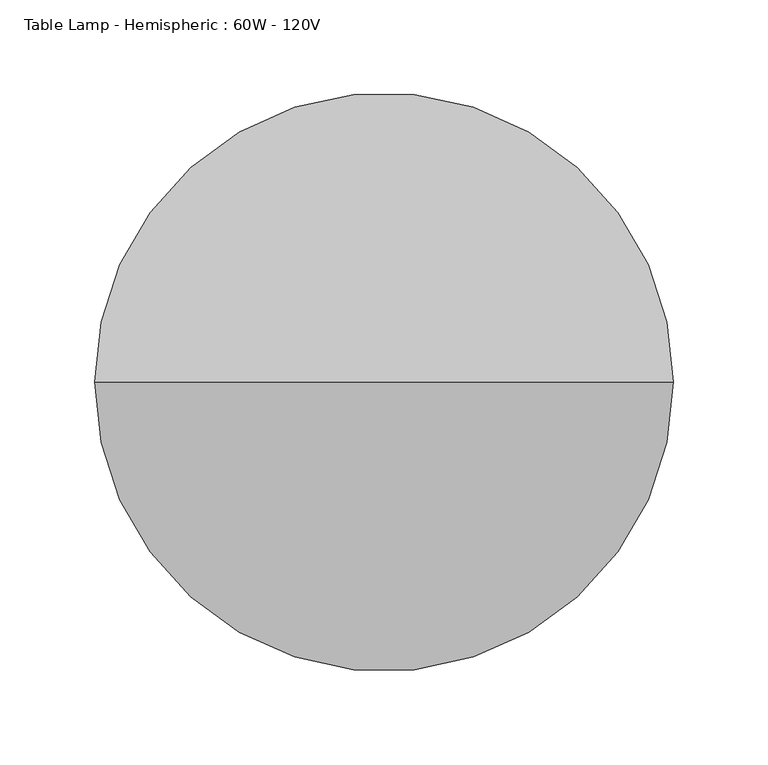
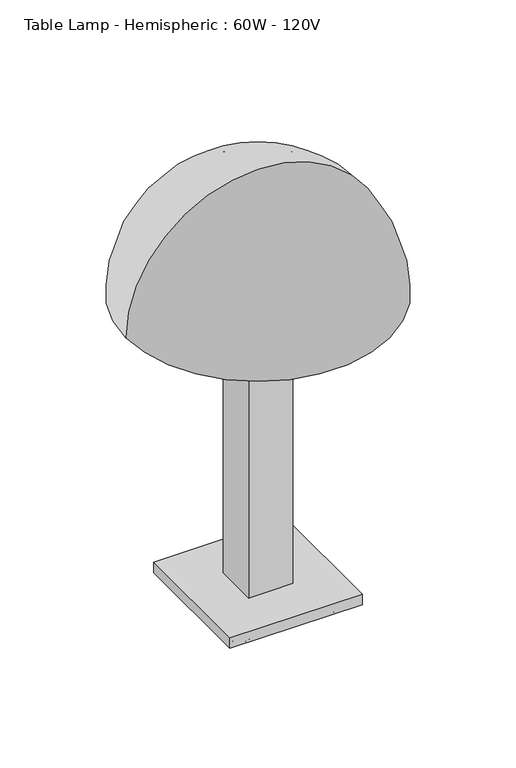
"""IFC4 building model written with IfcOpenShell, lengths in millimetres: light fixture geometry, Table Lamp - Hemispheric : 60W - 120V."""

from ifc_helpers import new_model, si_unit, point, frame, origin, origin_2d, place, context, project, spatial, polyline, circle_curve, ellipse_curve, trimmed, segment, composite_curve, outline, extrude, source, transform, mapped, element, save
from ifc_brep_helpers import plane_surface, revolved_surface, advanced_brep


def table_lamp_hemispheric_60w_120v_02721d88(model_context):
    return source(origin(), model_context, "Body", "SolidModel", [
        advanced_brep(
        [(0.0, 0.0, 524.5095504), (152.4, 0.0, 372.1095504), (-152.4, 0.0, 372.1095504), (-146.05, 0.0, 372.1095504), (146.05, 0.0, 372.1095504), (0.0, 0.0, 518.1595504)],
        [
            (0, 1, circle_curve(frame((0.0, 0.0, 372.1095504), z_axis=(0.0, 1.0, 0.0), x_axis=(1.0, 0.0, 0.0)), 152.4)),
            (1, 2, circle_curve(frame((0.0, 0.0, 372.1095504), z_axis=(0.0, 0.0, 1.0), x_axis=(1.0, 0.0, 0.0)), 152.4)),
            (2, 0, circle_curve(frame((0.0, 0.0, 372.1095504), z_axis=(0.0, 1.0, 0.0), x_axis=(-1.0, 0.0, 0.0)), 152.4)),
            (2, 1, circle_curve(frame((0.0, 0.0, 372.1095504), z_axis=(0.0, 0.0, 1.0), x_axis=(1.0, 0.0, 0.0)), 152.4)),
            (3, 4, circle_curve(frame((0.0, 0.0, 372.1095504), z_axis=(0.0, 0.0, -1.0), x_axis=(1.0, 0.0, 0.0)), 146.05)),
            (4, 5, circle_curve(frame((0.0, 0.0, 372.1095504), z_axis=(0.0, -1.0, 0.0), x_axis=(1.0, 0.0, 0.0)), 146.05)),
            (5, 3, circle_curve(frame((0.0, 0.0, 372.1095504), z_axis=(0.0, -1.0, 0.0), x_axis=(-1.0, 0.0, 0.0)), 146.05)),
            (4, 3, circle_curve(frame((0.0, 0.0, 372.1095504), z_axis=(0.0, 0.0, -1.0), x_axis=(1.0, 0.0, 0.0)), 146.05)),
            (1, 4),
            (3, 2),
        ],
        [
            revolved_surface(trimmed(ellipse_curve(frame((0.0, 0.0, 372.1095504), z_axis=(0.0, -1.0, 0.0), x_axis=(1.0, 0.0, 0.0)), 152.4, 152.4), [point((152.4, 0.0, 372.1095504))], [point((0.0, 0.0, 524.5095504))], True, "CARTESIAN"), (0.0, 0.0, 552.6321699), (0.0, 0.0, 1.0)),
            revolved_surface(trimmed(ellipse_curve(frame((0.0, 0.0, 372.1095504), z_axis=(0.0, 1.0, 0.0), x_axis=(1.0, 0.0, 0.0)), 146.05, 146.05), [point((0.0, 0.0, 518.1595504))], [point((146.05, 0.0, 372.1095504))], True, "CARTESIAN"), (0.0, 0.0, 552.6321699), (0.0, 0.0, 1.0)),
            plane_surface(frame((0.0, 0.0, 372.1095504), z_axis=(0.0, 0.0, -1.0), x_axis=(1.0, 0.0, 0.0))),
        ],
        [
            (0, [[1, 2, 3]]),
            (0, [[-3, 4, -1]]),
            (1, [[5, 6, 7]]),
            (1, [[8, -7, -6]]),
            (2, [[-2, 9, -5, 10]]),
            (2, [[-4, -10, -8, -9]]),
        ],
    ),
        extrude(outline(composite_curve([segment(trimmed(circle_curve(origin_2d(), 6.35), [point((-6.35, 0.0))], [point((6.35, 0.0))], False, "CARTESIAN"), True, "CONTINUOUS"), segment(trimmed(circle_curve(origin_2d(), 6.35), [point((6.35, 0.0))], [point((-6.35, 0.0))], False, "CARTESIAN"), True, "CONTINUOUS")], self_intersect=False)), frame((0.0, 0.0, 330.2), z_axis=(0.0, 0.0, 1.0), x_axis=(1.0, 0.0, 0.0)), (0.0, 0.0, 1.0), 63.5),
        extrude(outline(polyline([(25.4, -25.4), (-25.4, -25.4), (-25.4, 25.4), (25.4, 25.4), (25.4, -25.4)])), frame((0.0, 0.0, 25.4), z_axis=(0.0, 0.0, 1.0), x_axis=(1.0, 0.0, 0.0)), (0.0, 0.0, 1.0), 304.8),
        advanced_brep(
        [(-66.7336963, -50.8, 12.7), (-34.9836963, -50.8, 12.7), (-47.6836963, -50.8, 0.0), (-54.0336963, -50.8, 0.0), (-54.0336963, -50.8, 12.7), (-47.6836963, -50.8, 12.7)],
        [
            (0, 1, circle_curve(frame((-50.8586963, -50.8, 12.7), z_axis=(0.0, 0.0, -1.0), x_axis=(1.0, 0.0, 0.0)), 15.875)),
            (1, 2, circle_curve(frame((-47.6836963, -50.8, 12.7), z_axis=(0.0, 1.0, 0.0), x_axis=(1.0, 0.0, 0.0)), 12.7)),
            (2, 3, circle_curve(frame((-50.8586963, -50.8, 0.0), z_axis=(0.0, 0.0, 1.0), x_axis=(1.0, 0.0, 0.0)), 3.175)),
            (3, 0, circle_curve(frame((-54.0336963, -50.8, 12.7), z_axis=(0.0, 1.0, 0.0), x_axis=(-1.0, 0.0, 0.0)), 12.7)),
            (1, 0, circle_curve(frame((-50.8586963, -50.8, 12.7), z_axis=(0.0, 0.0, -1.0), x_axis=(1.0, 0.0, 0.0)), 15.875)),
            (3, 2, circle_curve(frame((-50.8586963, -50.8, 0.0), z_axis=(0.0, 0.0, 1.0), x_axis=(1.0, 0.0, 0.0)), 3.175)),
            (4, 5, circle_curve(frame((-50.8586963, -50.8, 12.7), z_axis=(0.0, 0.0, -1.0), x_axis=(1.0, 0.0, 0.0)), 3.175)),
            (5, 1),
            (0, 4),
            (5, 4, circle_curve(frame((-50.8586963, -50.8, 12.7), z_axis=(0.0, 0.0, -1.0), x_axis=(1.0, 0.0, 0.0)), 3.175)),
            (2, 5),
            (4, 3),
        ],
        [
            revolved_surface(trimmed(ellipse_curve(frame((-47.6836963, -50.8, 12.7), z_axis=(0.0, -1.0, 0.0), x_axis=(1.0, 0.0, 0.0)), 12.7, 12.7), [point((-47.6836963, -50.8, 0.0))], [point((-34.9836963, -50.8, 12.7))], True, "CARTESIAN"), (-50.8586963, -50.8, 36.0623287), (0.0, 0.0, 1.0)),
            plane_surface(frame((-50.8586963, -50.8, 12.7), z_axis=(0.0, 0.0, 1.0), x_axis=(1.0, 0.0, 0.0))),
            revolved_surface(polyline([(-47.6836963, -50.8, 12.7), (-47.6836963, -50.8, 0.0)]), (-50.8586963, -50.8, 36.0623287), (0.0, 0.0, 1.0)),
        ],
        [
            (0, [[1, 2, 3, 4]]),
            (0, [[5, -4, 6, -2]]),
            (1, [[7, 8, -1, 9]]),
            (1, [[10, -9, -5, -8]]),
            (2, [[-3, 11, -7, 12]]),
            (2, [[-6, -12, -10, -11]]),
        ],
    ),
        advanced_brep(
        [(-66.7581301, 50.8, 12.7), (-35.0081301, 50.8, 12.7), (-47.7081301, 50.8, 0.0), (-54.0581301, 50.8, 0.0), (-54.0581301, 50.8, 12.7), (-47.7081301, 50.8, 12.7)],
        [
            (0, 1, circle_curve(frame((-50.8831301, 50.8, 12.7), z_axis=(0.0, 0.0, -1.0), x_axis=(1.0, 0.0, 0.0)), 15.875)),
            (1, 2, circle_curve(frame((-47.7081301, 50.8, 12.7), z_axis=(0.0, 1.0, 0.0), x_axis=(1.0, 0.0, 0.0)), 12.7)),
            (2, 3, circle_curve(frame((-50.8831301, 50.8, 0.0), z_axis=(0.0, 0.0, 1.0), x_axis=(1.0, 0.0, 0.0)), 3.175)),
            (3, 0, circle_curve(frame((-54.0581301, 50.8, 12.7), z_axis=(0.0, 1.0, 0.0), x_axis=(-1.0, 0.0, 0.0)), 12.7)),
            (1, 0, circle_curve(frame((-50.8831301, 50.8, 12.7), z_axis=(0.0, 0.0, -1.0), x_axis=(1.0, 0.0, 0.0)), 15.875)),
            (3, 2, circle_curve(frame((-50.8831301, 50.8, 0.0), z_axis=(0.0, 0.0, 1.0), x_axis=(1.0, 0.0, 0.0)), 3.175)),
            (4, 5, circle_curve(frame((-50.8831301, 50.8, 12.7), z_axis=(0.0, 0.0, -1.0), x_axis=(1.0, 0.0, 0.0)), 3.175)),
            (5, 1),
            (0, 4),
            (5, 4, circle_curve(frame((-50.8831301, 50.8, 12.7), z_axis=(0.0, 0.0, -1.0), x_axis=(1.0, 0.0, 0.0)), 3.175)),
            (2, 5),
            (4, 3),
        ],
        [
            revolved_surface(trimmed(ellipse_curve(frame((-47.7081301, 50.8, 12.7), z_axis=(0.0, -1.0, 0.0), x_axis=(1.0, 0.0, 0.0)), 12.7, 12.7), [point((-47.7081301, 50.8, 0.0))], [point((-35.0081301, 50.8, 12.7))], True, "CARTESIAN"), (-50.8831301, 50.8, 36.0623287), (0.0, 0.0, 1.0)),
            plane_surface(frame((-50.8831301, 50.8, 12.7), z_axis=(0.0, 0.0, 1.0), x_axis=(1.0, 0.0, 0.0))),
            revolved_surface(polyline([(-47.708130100000005, 50.8, 12.7), (-47.708130100000005, 50.8, 0.0)]), (-50.8831301, 50.8, 36.0623287), (0.0, 0.0, 1.0)),
        ],
        [
            (0, [[1, 2, 3, 4]]),
            (0, [[5, -4, 6, -2]]),
            (1, [[7, 8, -1, 9]]),
            (1, [[10, -9, -5, -8]]),
            (2, [[-3, 11, -7, 12]]),
            (2, [[-6, -12, -10, -11]]),
        ],
    ),
        advanced_brep(
        [(34.9494337, -50.8, 12.7), (66.6994337, -50.8, 12.7), (53.9994337, -50.8, 0.0), (47.6494337, -50.8, 0.0), (47.6494337, -50.8, 12.7), (53.9994337, -50.8, 12.7)],
        [
            (0, 1, circle_curve(frame((50.8244337, -50.8, 12.7), z_axis=(0.0, 0.0, -1.0), x_axis=(1.0, 0.0, 0.0)), 15.875)),
            (1, 2, circle_curve(frame((53.9994337, -50.8, 12.7), z_axis=(0.0, 1.0, 0.0), x_axis=(1.0, 0.0, 0.0)), 12.7)),
            (2, 3, circle_curve(frame((50.8244337, -50.8, 0.0), z_axis=(0.0, 0.0, 1.0), x_axis=(1.0, 0.0, 0.0)), 3.175)),
            (3, 0, circle_curve(frame((47.6494337, -50.8, 12.7), z_axis=(0.0, 1.0, 0.0), x_axis=(-1.0, 0.0, 0.0)), 12.7)),
            (1, 0, circle_curve(frame((50.8244337, -50.8, 12.7), z_axis=(0.0, 0.0, -1.0), x_axis=(1.0, 0.0, 0.0)), 15.875)),
            (3, 2, circle_curve(frame((50.8244337, -50.8, 0.0), z_axis=(0.0, 0.0, 1.0), x_axis=(1.0, 0.0, 0.0)), 3.175)),
            (4, 5, circle_curve(frame((50.8244337, -50.8, 12.7), z_axis=(0.0, 0.0, -1.0), x_axis=(1.0, 0.0, 0.0)), 3.175)),
            (5, 1),
            (0, 4),
            (5, 4, circle_curve(frame((50.8244337, -50.8, 12.7), z_axis=(0.0, 0.0, -1.0), x_axis=(1.0, 0.0, 0.0)), 3.175)),
            (2, 5),
            (4, 3),
        ],
        [
            revolved_surface(trimmed(ellipse_curve(frame((53.9994337, -50.8, 12.7), z_axis=(0.0, -1.0, 0.0), x_axis=(1.0, 0.0, 0.0)), 12.7, 12.7), [point((53.9994337, -50.8, 0.0))], [point((66.6994337, -50.8, 12.7))], True, "CARTESIAN"), (50.8244337, -50.8, 36.0623287), (0.0, 0.0, 1.0)),
            plane_surface(frame((50.8244337, -50.8, 12.7), z_axis=(0.0, 0.0, 1.0), x_axis=(1.0, 0.0, 0.0))),
            revolved_surface(polyline([(53.9994337, -50.8, 12.7), (53.9994337, -50.8, 0.0)]), (50.8244337, -50.8, 36.0623287), (0.0, 0.0, 1.0)),
        ],
        [
            (0, [[1, 2, 3, 4]]),
            (0, [[5, -4, 6, -2]]),
            (1, [[7, 8, -1, 9]]),
            (1, [[10, -9, -5, -8]]),
            (2, [[-3, 11, -7, 12]]),
            (2, [[-6, -12, -10, -11]]),
        ],
    ),
        advanced_brep(
        [(34.925, 50.8, 12.7), (66.675, 50.8, 12.7), (53.975, 50.8, 0.0), (47.625, 50.8, 0.0), (47.625, 50.8, 12.7), (53.975, 50.8, 12.7)],
        [
            (0, 1, circle_curve(frame((50.8, 50.8, 12.7), z_axis=(0.0, 0.0, -1.0), x_axis=(1.0, 0.0, 0.0)), 15.875)),
            (1, 2, circle_curve(frame((53.975, 50.8, 12.7), z_axis=(0.0, 1.0, 0.0), x_axis=(1.0, 0.0, 0.0)), 12.7)),
            (2, 3, circle_curve(frame((50.8, 50.8, 0.0), z_axis=(0.0, 0.0, 1.0), x_axis=(1.0, 0.0, 0.0)), 3.175)),
            (3, 0, circle_curve(frame((47.625, 50.8, 12.7), z_axis=(0.0, 1.0, 0.0), x_axis=(-1.0, 0.0, 0.0)), 12.7)),
            (1, 0, circle_curve(frame((50.8, 50.8, 12.7), z_axis=(0.0, 0.0, -1.0), x_axis=(1.0, 0.0, 0.0)), 15.875)),
            (3, 2, circle_curve(frame((50.8, 50.8, 0.0), z_axis=(0.0, 0.0, 1.0), x_axis=(1.0, 0.0, 0.0)), 3.175)),
            (4, 5, circle_curve(frame((50.8, 50.8, 12.7), z_axis=(0.0, 0.0, -1.0), x_axis=(1.0, 0.0, 0.0)), 3.175)),
            (5, 1),
            (0, 4),
            (5, 4, circle_curve(frame((50.8, 50.8, 12.7), z_axis=(0.0, 0.0, -1.0), x_axis=(1.0, 0.0, 0.0)), 3.175)),
            (2, 5),
            (4, 3),
        ],
        [
            revolved_surface(trimmed(ellipse_curve(frame((53.975, 50.8, 12.7), z_axis=(0.0, -1.0, 0.0), x_axis=(1.0, 0.0, 0.0)), 12.7, 12.7), [point((53.975, 50.8, 0.0))], [point((66.675, 50.8, 12.7))], True, "CARTESIAN"), (50.8, 50.8, 36.0623287), (0.0, 0.0, 1.0)),
            plane_surface(frame((50.8, 50.8, 12.7), z_axis=(0.0, 0.0, 1.0), x_axis=(1.0, 0.0, 0.0))),
            revolved_surface(polyline([(53.974999999999994, 50.8, 12.7), (53.974999999999994, 50.8, 0.0)]), (50.8, 50.8, 36.0623287), (0.0, 0.0, 1.0)),
        ],
        [
            (0, [[1, 2, 3, 4]]),
            (0, [[5, -4, 6, -2]]),
            (1, [[7, 8, -1, 9]]),
            (1, [[10, -9, -5, -8]]),
            (2, [[-3, 11, -7, 12]]),
            (2, [[-6, -12, -10, -11]]),
        ],
    ),
        extrude(outline(polyline([(76.2, 76.2), (76.2, -76.2), (-76.2, -76.2), (-76.2, 76.2), (76.2, 76.2)])), frame((0.0, 0.0, 12.7), z_axis=(0.0, 0.0, 1.0), x_axis=(1.0, 0.0, 0.0)), (0.0, 0.0, 1.0), 12.7),
    ])


if __name__ == "__main__":
    model = new_model("IFC4")
    model_context = context("Model", 3, world=origin())
    ifc_project = project(units=[si_unit("LENGTHUNIT", "METRE", prefix="MILLI")], contexts=[model_context])
    site = spatial("IfcSite", under=ifc_project)
    building = spatial("IfcBuilding", under=site)
    placement = place(None, origin())
    table_lamp_hemispheric_60w_120v_shape = table_lamp_hemispheric_60w_120v_02721d88(model_context)
    element("IfcLightFixture", 1, ObjectType="Table Lamp - Hemispheric : 60W - 120V", at=placement, inside=building, context=model_context, shape_type="MappedRepresentation", body=[
        mapped(table_lamp_hemispheric_60w_120v_shape, transform((0.0, 0.0, 0.0), x_axis=(1.0, 0.0, 0.0), y_axis=(0.0, 1.0, 0.0), z_axis=(0.0, 0.0, 1.0))),
    ])
    save(model, "model.ifc")

# Revit data of these elements
# Type "Table Lamp - Hemispheric : 60W - 120V"
#   Assembly Code = "D5020220"
#   Lamp = "A-19"
#   Wattage = 60 W
#   built-in parameter 1150110 = 1 (stored number, unit not read)
#   built-in parameter 1114217 = 1 (stored number, unit not read)
#   built-in parameter 1150109 = 1 (stored number, unit not read)
#   built-in parameter 1150113 = 1 (stored number, unit not read)
#   built-in parameter 1150115 = 1 (stored number, unit not read)
#   built-in parameter 1150105 = 68.0387 (stored number, unit not read)
#   Light Source Symbol Size = 2' - 0"
#   built-in parameter 1150112 = 1 (stored number, unit not read)
#   built-in parameter 1150114 = 1 (stored number, unit not read)
#   built-in parameter 1150107 = 2800 (stored number, unit not read)
#   built-in parameter 1150106 = 0.680387 (stored number, unit not read)
#   built-in parameter 1150104 = 1.32387 (stored number, unit not read)
#   Ballast Voltage = 120 V
#   built-in parameter 1114218 = 1 (stored number, unit not read)
#   built-in parameter 1150133 = 10 (stored number, unit not read)
#   Lumens = 855 lm
#   Apparent Load = 60 VA
#   built-in parameter 1150134 = 4
#   built-in parameter 1150137 = 1
#   Color Filter = 16777215
#   Ballast Number of Poles = 1
#   Mount Material = Steel, Chrome Plated
#   Shade Material = Glass, Frosted
#   Base Material = Birch
#   Dimming Lamp Color Temperature Shift = (empty or 0)
#   Wattage Comments = ""
# Element 1 (IfcLightFixture, "Table Lamp - Hemispheric : 60W - 120V")
#   Materials on its faces: "Steel, Chrome Plated", "Glass, Frosted", "Birch"
# Materials
#   "Steel, Chrome Plated": class "Metal", colour RGB 17 17 17, transparency 0, Description = "Chromiuim plated steel", Cost = 0
#   "Glass, Frosted": class "Glass", colour RGB 250 244 225, transparency 0.55, Description = "physical material", Cost = 0
#   "Birch": class "Wood", colour RGB 224 178 126, transparency 0, Description = "Betula Alleghaniensis", Cost = 0
